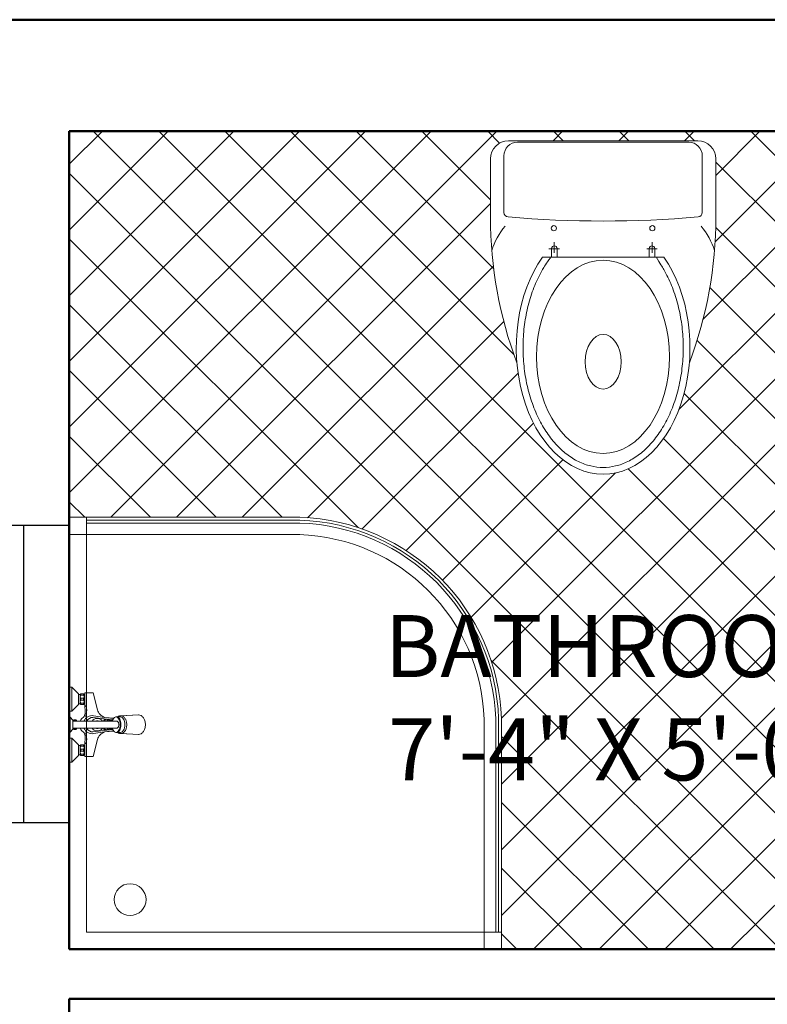
# Model space of a CAD drawing. Units: inches. Extents: x -466983 to 1020, y 324 to 318697.
# Tile 97 of 97: x 810 to 870, y 1006 to 1085. Entities that reach past the tile are written whole.
import ezdxf

# ---------------------------------------------------------------- set-up
doc = ezdxf.new("R2010")
doc.units = ezdxf.units.IN
doc.header["$MEASUREMENT"] = 0
for name, color, linetype, lineweight in [('A-AREA-IDEN', 7, 'Continuous', 25), ('A-FLOR-FIXT', 9, 'Continuous', 18), ('A-FLOR-PATT', 252, 'Continuous', 13), ('A-GLAZ', 4, 'Continuous', 25), ('A-WALL', 7, 'Continuous', 50)]:
    doc.layers.add(name, color=color, linetype=linetype, lineweight=lineweight)
doc.styles.get("Standard").update_dxf_attribs({"font": 'arial.ttf'})

# ---------------------------------------------------------------- blocks, each defined once
blk = doc.blocks.new('Ventilator')
for p, q in [((1433.5927409432, 801.6799676286266), (1457.592740943201, 801.6799676286266)), ((1433.5927409432, 792.6799676286266), (1433.5927409432, 801.6799676286266)), ((1457.592740943201, 801.6799676286266), (1457.592740943201, 792.6799676286266)), ((1433.5927409432, 797.9799676286265), (1457.592740943201, 797.9799676286265)), ((1457.592740943201, 796.3799676286266), (1433.5927409432, 796.3799676286266)), ((1457.592740943201, 792.6799676286266), (1433.5927409432, 792.6799676286266))]:
    blk.add_line(p, q)
blk = doc.blocks.new('B1')
for p, q in [((0, 1300.000000000277), (693.3333333334303, 1300.000000000277)), ((0, 1.023182e-10), (0, 1300.000000000277)), ((52.00000000000727, 52.00000000000045), (52.00000000000727, 1300.000000000277)), ((52.00000000000727, 1291.33333333362), (693.3333333334303, 1291.33333333362)), ((52.00000000000727, 1282.666666666948), (693.3333333334303, 1282.666666666948)), ((0, 1248.000000000277), (693.3333333334303, 1248.000000000277)), ((21.99999999999818, 689.0000000001346), (21.99999999999818, 687.0000000001382)), ((140.3876720592416, 699.4289321882679), (154.4144116848583, 699.4289321882679)), ((208.8876720592416, 705.4289321882679), (153.4804125083301, 702.8756022550479)), ((1248.000000000174, 693.6609680139231), (1248.000000000174, 1.023182e-10)), ((1282.666666666846, 693.6609680139231), (1282.666666666846, 52.00000000010231)), ((1291.333333333514, 693.6609680139231), (1291.333333333517, 52.00000000010231)), ((1300.000000000182, 693.6609680139231), (1300.000000000182, 1.023182e-10)), ((21.99999999999818, 663.0000000001382), (21.99999999999818, 665.0000000001309)), ((140.3876720592416, 652.5710678120049), (154.4144116848583, 652.5710678120049)), ((208.8876720592416, 646.5710678120049), (153.5459520445456, 648.976381547378)), ((52.00000000001091, 52.00000000000045), (1300.000000000178, 52.00000000010231)), ((0, 4.547e-13), (1300.000000000182, 1.023182e-10))]:
    blk.add_line(p, q)
for points in [[(0, 775.000000000131), (0, 789.0000000001346), (8, 789.0000000001346)], [(0, 754.0000000001382), (0, 775.000000000131)], [(8, 789.0000000001346), (8, 717.0000000001309)], [(8, 789.0000000001346), (27.99999999999818, 769.0000000001309), (27.99999999999818, 767.0000000001382)], [(8, 717.0000000001309), (0, 717.0000000001309), (0, 754.0000000001382)], [(27.99999999999818, 767.0000000001382), (33.00000000000182, 767.0000000001382)], [(27.99999999999818, 767.0000000001382), (27.99999999999818, 753.0000000001345)], [(27.99999999999818, 739.0000000001382), (27.99999999999818, 753.0000000001345)], [(33.00000000000182, 767.0000000001382), (35, 769.0000000001309), (43, 769.0000000001309), (45.00000000000182, 767.0000000001382)], [(33.00000000000182, 767.0000000001382), (33.00000000000182, 753.0000000001345)], [(35, 765.0000000001345), (33.00000000000182, 762.0000000001346)], [(33.00000000000182, 758.0000000001346), (35, 756.0000000001346), (43, 756.0000000001346), (45.00000000000182, 758.0000000001346)], [(33.00000000000182, 739.0000000001382), (33.00000000000182, 753.0000000001345)], [(33.00000000000182, 748.0000000001382), (35, 750.0000000001346), (43, 750.0000000001346), (45.00000000000182, 748.0000000001382)], [(35, 741.0000000001346), (33.00000000000182, 744.0000000001345)], [(43, 769.0000000001309), (43, 765.0000000001345), (35, 765.0000000001345), (35, 769.0000000001309)], [(35, 756.0000000001346), (35, 753.0000000001345)], [(35, 750.0000000001346), (35, 753.0000000001345)], [(43, 737.0000000001346), (43, 741.0000000001346), (35, 741.0000000001346), (35, 737.0000000001346)], [(43, 765.0000000001345), (45.00000000000182, 763.0000000001382)], [(43, 756.0000000001346), (43, 753.0000000001345)], [(43, 750.0000000001346), (43, 753.0000000001345)], [(43, 741.0000000001346), (45.00000000000182, 743.0000000001346)], [(47, 767.0000000001382), (45.00000000000182, 767.0000000001382)], [(45.00000000000182, 767.0000000001382), (45.00000000000182, 753.0000000001345)], [(45.00000000000182, 739.0000000001382), (45.00000000000182, 753.0000000001345)], [(47, 739.0000000001382), (47, 767.0000000001382)], [(8, 717.0000000001309), (27.99999999999818, 737.0000000001346), (27.99999999999818, 739.0000000001382)], [(27.99999999999818, 739.0000000001382), (33.00000000000182, 739.0000000001382)], [(33.00000000000182, 739.0000000001382), (35, 737.0000000001346), (43, 737.0000000001346), (45.00000000000182, 739.0000000001382)], [(47, 739.0000000001382), (45.00000000000182, 739.0000000001382)], [(47, 728.0000000001345), (47, 739.0000000001382)], [(0, 687.0000000001382), (0, 699.0000000001382)], [(0, 699.0000000001382), (3, 699.0000000001382)], [(0, 665.0000000001309), (0, 687.0000000001382)], [(3, 699.0000000001382), (3, 676.0000000001346)], [(3, 699.0000000001382), (11, 690.0000000001382), (11, 687.0000000001382)], [(11, 687.0000000001382), (11, 676.0000000001346)], [(140.9999999999982, 687.0000000001382), (11, 687.0000000001382)], [(0, 653.0000000001309), (0, 665.0000000001309)], [(0, 653.0000000001309), (3, 653.0000000001309)], [(3, 653.0000000001309), (3, 676.0000000001346)], [(3, 653.0000000001309), (11, 662.000000000131), (11, 665.0000000001309)], [(11, 665.0000000001309), (11, 676.0000000001346)], [(140.9999999999982, 665.0000000001309), (11, 665.0000000001309)], [(133.9221670278657, 656.0563042479444), (133.0620831697051, 656.0563042479444)], [(7.999999999998181, 635.0000000001382), (0, 635.0000000001382), (0, 598.0000000001309)], [(7.999999999998181, 563.0000000001346), (7.999999999998181, 635.0000000001382)], [(7.999999999998181, 635.0000000001382), (27.99999999999818, 615.0000000001345), (27.99999999999818, 613.0000000001346)], [(47, 624.0000000001345), (47, 613.0000000001346)], [(0, 598.0000000001309), (0, 577.0000000001382)], [(27.99999999999818, 613.0000000001346), (27.99999999999818, 599.0000000001382)], [(27.99999999999818, 613.0000000001346), (33.00000000000182, 613.0000000001346)], [(27.99999999999818, 585.0000000001346), (27.99999999999818, 599.0000000001382)], [(33.00000000000182, 613.0000000001346), (35, 615.0000000001345), (42.99999999999818, 615.0000000001345), (45.00000000000182, 613.0000000001346)], [(33.00000000000182, 613.0000000001346), (33.00000000000182, 599.0000000001382)], [(35, 611.0000000001382), (33.00000000000182, 608.0000000001382)], [(33.00000000000182, 604.0000000001346), (35, 602.0000000001382), (42.99999999999818, 602.0000000001382), (45.00000000000182, 604.0000000001346)], [(33.00000000000182, 585.0000000001346), (33.00000000000182, 599.0000000001382)], [(33.00000000000182, 594.0000000001345), (35, 596.0000000001382), (42.99999999999818, 596.0000000001382), (45.00000000000182, 594.0000000001345)], [(42.99999999999818, 615.0000000001345), (42.99999999999818, 611.0000000001382), (35, 611.0000000001382), (35, 615.0000000001345)], [(35, 602.0000000001382), (35, 599.0000000001382)], [(35, 596.0000000001382), (35, 599.0000000001382)], [(42.99999999999818, 611.0000000001382), (45.00000000000182, 609.0000000001346)], [(42.99999999999818, 602.0000000001382), (42.99999999999818, 599.0000000001382)], [(42.99999999999818, 596.0000000001382), (42.99999999999818, 599.0000000001382)], [(45.00000000000182, 613.0000000001346), (45.00000000000182, 599.0000000001382)], [(47, 613.0000000001346), (45.00000000000182, 613.0000000001346)], [(45.00000000000182, 585.0000000001346), (45.00000000000182, 599.0000000001382)], [(47, 613.0000000001346), (47, 585.0000000001346)], [(0, 577.0000000001382), (0, 563.0000000001346), (7.999999999998181, 563.0000000001346)], [(7.999999999998181, 563.0000000001346), (27.99999999999818, 583.000000000131), (27.99999999999818, 585.0000000001346)], [(27.99999999999818, 585.0000000001346), (33.00000000000182, 585.0000000001346)], [(35, 587.0000000001382), (33.00000000000182, 590.0000000001382)], [(33.00000000000182, 585.0000000001346), (35, 583.000000000131), (42.99999999999818, 583.000000000131), (45.00000000000182, 585.0000000001346)], [(42.99999999999818, 583.000000000131), (42.99999999999818, 587.0000000001382), (35, 587.0000000001382), (35, 583.000000000131)], [(42.99999999999818, 587.0000000001382), (45.00000000000182, 589.0000000001309)], [(47, 585.0000000001346), (45.00000000000182, 585.0000000001346)]]:
    blk.add_lwpolyline(points)
blk.add_lwpolyline([(208.8876720592416, 646.5710678120049), (154.6376720593016, 648.9289321882679, -0.1383183006310921), (148.063043746286, 650.7831906028294, -0.0370381408635636), (145.578855038857, 652.5710678120049), (140.3876720592379, 652.5710678120049, -0.1665558057867227), (136.092755137337, 654.0425753596318, -0.0535717192020755), (133.4948936773198, 656.547585930646), (107, 654.0000000001382, 0.2625940722123521), (85, 631.0000000001346), (72, 580.0000000001419), (47, 580.0000000001419), (47, 585.0000000001346), (45.00000000000182, 585.0000000001346), (42.99999999999818, 583.0000000001346), (35, 583.0000000001346), (33.00000000000182, 585.0000000001346), (27.99999999999818, 585.0000000001346), (27.99999999999818, 583.0000000001346), (7.999999999998181, 563.0000000001382), (0, 563.0000000001382), (0, 577.0000000001418), (0, 598.0000000001346), (0, 635.0000000001418), (7.999999999998181, 635.0000000001418), (27.99999999999818, 615.0000000001382), (27.99999999999818, 613.0000000001346), (33.00000000000182, 613.0000000001346), (35, 615.0000000001382), (42.99999999999818, 615.0000000001382), (45.00000000000182, 613.0000000001346), (47, 613.0000000001346), (47, 624.0000000001382, 0.1247866838288863), (46, 648.0000000001382, 0.1501483781683498), (42.00000000000182, 654.0000000001382, -0.1384844099870248), (32.50754085593508, 665.0000000001345), (21.99999999999818, 665.0000000001345), (21.99999999999818, 663.0000000001382, -0.3003468456066685), (11, 662.3397459768711), (11, 662.0000000001346), (3, 653.0000000001345), (0, 653.0000000001345), (0, 665.0000000001345), (0, 687.0000000001382), (0, 699.0000000001418), (3, 699.0000000001418), (11, 690.0000000001382), (10.99999999999636, 689.6602540496569, -0.3003468456580443), (21.99999999999818, 689.0000000001346), (21.99999999999818, 687.0000000001382), (32.50754085593508, 687.0000000001382, -0.138484409987018), (42.00000000000182, 698.0000000001346, 0.1501483781683498), (46, 704.0000000001346, 0.1247866838288863), (47, 728.0000000001382), (47, 739.0000000001382), (45.00000000000182, 739.0000000001382), (43, 737.0000000001382), (35, 737.0000000001382), (33.00000000000182, 739.0000000001382), (27.99999999999818, 739.0000000001382), (27.99999999999818, 737.0000000001382), (8, 717.0000000001346), (0, 717.0000000001346), (0, 754.0000000001382), (0, 775.0000000001346), (0, 789.0000000001382), (8, 789.0000000001382), (27.99999999999818, 769.0000000001345), (27.99999999999818, 767.0000000001382), (33.00000000000182, 767.0000000001382), (35, 769.0000000001345), (43, 769.0000000001345), (45.00000000000182, 767.0000000001382), (47, 767.0000000001382), (47, 772.0000000001346), (72, 772.0000000001346), (85, 721.0000000001382, 0.2625940722123521), (107, 698.0000000001346), (133.494893670435, 695.4524140702815, -0.0535717192022979), (136.092755137337, 697.9574246406409, -0.1665558057868109), (140.3876720592416, 699.4289321882679), (145.7502000114491, 699.4289321882679, -0.0343443404771406), (148.063043746286, 701.07467377371, -0.1383183006298331), (154.6376720592416, 702.9289321882715), (208.8876720591488, 705.4289321882679, -0.1377032461334603), (216.0999264221609, 703.4042378869926, -0.1070360850488126), (223.0298076829695, 696.809397513447, -0.0808015121757586), (227.273223711496, 687.6931912444343, -0.0687078013104136), (228.8876720592398, 676.0000000001382, -0.0687078013104135), (227.273223711496, 664.3068087558385, -0.0808015121757595), (223.0298076829695, 655.1906024868258, -0.107036085048811), (216.0999264221609, 648.5957621132802, -0.1377032461317454)], format="xyb", close=True)
for points in [[(47, 767.0000000001382), (47, 772.0000000001309), (72, 772.0000000001309), (85, 721.0000000001382, 0.2625940722123521), (107, 698.0000000001346), (133.4948936704422, 695.4524140702887, -0.3591123035969264)], [(47, 728.0000000001345, -0.1247866838288863), (46, 704.0000000001346, -0.1501483781683498), (42.00000000000182, 698.0000000001346, 0.138484409987018), (32.50754085593508, 687.0000000001382, 0.7633705308853952)], [(47, 734.0000000001346, -0.2052577019546359), (52, 726.0000000001309, -0.1374236490949136), (49, 701.0000000001346, -5.029096516974528)], [(11, 688.0000000001346, -0.2034527507076884), (11.27314869702968, 688.6434964536201, -0.0971632324952149), (12.46446609406666, 689.4142135625043, -0.0541309211895364), (13.96123847455419, 689.8322469457524, -0.041071521782227), (15.99999999999818, 690.0000000001382, -0.041071521782232), (18.03876152544581, 689.8322469457524, -0.0541309211895581), (19.53553390593333, 689.4142135625043, -0.0971632324952149), (20.72685130297032, 688.6434964536201, -0.2034527507076884), (21, 688.0000000001346, -0.2034527507076693), (20.72685130297032, 687.3565035466526, -0.0379533313060429), (20.29672106629732, 687.0000000001382, -0.0541309211895384)], [(11.70327893370086, 687.0000000001382, -0.0379533313059558), (11.27314869702968, 687.3565035466526, -0.2034527507076722), (11, 688.0000000001346, -0.2034527507076884)], [(11.14357068821118, 689.7415727613479, -0.2958552022276962), (21.99999999999818, 689.0000000001346, -2.290285352134018)], [(106.0000000000018, 698.0000000001346), (73, 703.0000000001382, 0.3410628393219512), (44.19402075297876, 687.0000000001382, 0.987420997957196)], [(71.00000000000182, 698.0000000001346, 0.2653451188970793), (52.73167562087656, 687.0000000001382, 0.6855978624637613)], [(71.00000000000182, 698.0000000001346), (130.3767751999166, 690.0830966401517, -0.389881551935721)], [(109.0000000000018, 693.0000000001382, 0.3394066855219726), (103.0542662941007, 687.0000000001382)], [(105.3371881863113, 687.0000000001382, -0.2701562118716146), (110, 691.0000000001346), (129.6983785438242, 688.2641140912746, -0.3982822486971544)], [(106.0000000000018, 698.0000000001346), (132.9051195245556, 694.7054955685562, -0.3445125279727503)], [(129.2869436463206, 665.0799945585786, 0.0546118951167688), (131.5488372944073, 659.4332431739494, 0.1055200220071626), (136.092755137337, 654.0425753596318, 0.1665558057868128), (140.3876720592416, 652.5710678120049, 0.1665558057868108), (144.6825889811407, 654.0425753596318, 0.1055200220071628), (149.2265068240704, 659.4332431739494, 0.0682582856346859), (151.8562849435693, 666.5533485092964, 0.0544283700167335), (152.8876720592398, 676.0000000001346, 0.0544283700167333), (151.8562849435693, 685.4466514909764, 0.0682582856346864), (149.2265068240704, 692.5667568263307, 0.1055200220071624), (144.6825889811407, 697.9574246406409, 0.1665558057868127), (140.3876720592416, 699.4289321882679, 0.1665558057868109), (136.092755137337, 697.9574246406409, 0.1055200220071607), (131.5488372944073, 692.5667568263307, 0.0538660454735237), (129.3093729212014, 687.0000000001382, 0.0544283700167342)], [(140.9999999999982, 665.0000000001309, 0.130158640187584), (143.919967274478, 665.7732172227988, 0.1064685849763611), (146.6568542494933, 668.2218254070867, 0.0842476149744631), (148.3593095850538, 671.6519929664936, 0.0732806852421333), (149, 676.0000000001346, 0.0732806852421325), (148.3593095850538, 680.3480070337755, 0.0842476149744645), (146.6568542494933, 683.7781745931861, 0.1064685849763632), (143.919967274478, 686.226782777474, 0.1301586401875921), (140.9999999999982, 687.0000000001382, 0.1301586401875932)], [(141.6455361051521, 652.6849517968694, 0.0451764077839428), (142.9034001510663, 652.5710678120049, 0.1665558057868108), (147.1983170729654, 654.0425753596318, 0.1055200220071628), (151.7422349158969, 659.4332431739494, 0.0682582856346859), (154.3720130353958, 666.5533485092964, 0.0544283700167335), (155.4034001510663, 676.0000000001346, 0.0544283700167333), (154.3720130353958, 685.4466514909764, 0.0682582856346864), (151.7422349158969, 692.5667568263307, 0.1055200220071624), (147.1983170729654, 697.9574246406409, 0.1665558057868127), (142.9034001510663, 699.4289321882679, 0.0451764077839423), (141.6455361051521, 699.315048203407, 0.1055200220071607)], [(145.5788550388533, 652.5710678120049, 0.0370381408635636), (148.063043746286, 650.7831906028294, 0.1383183006298338), (154.6376720592416, 648.9289321882679, 0.138318300629834), (161.2123003721917, 650.7831906028294, 0.1070627939593127), (167.5423708158942, 656.8370490962297, 0.0805227312927088), (171.4136097265637, 665.1966168081926, 0.0683531574638633), (172.8876720592398, 675.9289321882679, 0.0683531574638646), (171.4136097265637, 686.6612475683432, 0.0805227312927094), (167.5423708158942, 695.0208152803061, 0.1070627939593105), (161.2123003721917, 701.07467377371, 0.1383183006298341), (154.6376720592416, 702.9289321882715, 0.1383183006298331), (148.063043746286, 701.07467377371, 0.0343443404771406), (145.7502000114491, 699.4289321882679, 0.0805227312927093)], [(154.4144116848583, 652.5710678120049, 0.1665558057868108), (158.7093286067611, 654.0425753596318, 0.1055200220071628), (163.2532464496908, 659.4332431739494, 0.0682582856346859), (165.8830245691897, 666.5533485092964, 0.0544283700167335), (166.9144116848601, 676.0000000001346, 0.0544283700167333), (165.8830245691897, 685.4466514909764, 0.0682582856346864), (163.2532464496908, 692.5667568263307, 0.1055200220071624), (158.7093286067611, 697.9574246406409, 0.1665558057868127), (154.4144116848583, 699.4289321882679, 0.1665558057868109)], [(207.6853336958775, 646.6233249695179, 0.0217212157548433), (208.8876720592416, 646.5710678120049, 0.1377032461317454), (216.0999264221609, 648.5957621132802, 0.107036085048811), (223.0298076829695, 655.1906024868258, 0.0808015121757595), (227.273223711496, 664.3068087558385, 0.0687078013104135), (228.8876720592398, 676.0000000001346, 0.0687078013104136), (227.273223711496, 687.6931912444343, 0.0808015121757586), (223.0298076829695, 696.809397513447, 0.1070360850488126), (216.0999264221609, 703.4042378869926, 0.1377032461317515), (208.8876720592416, 705.4289321882679, 0.0115815460008583), (208.2459469633304, 705.4140658567775, 0.1070360850488107)], [(11, 664.0000000001346, 0.2034527507076884), (11.27314869702968, 663.356503546649, 0.0971632324952149), (12.46446609406666, 662.5857864377649, 0.0541309211895364), (13.96123847455419, 662.1677530545167, 0.041071521782227), (15.99999999999818, 662.000000000131, 0.041071521782232), (18.03876152544581, 662.1677530545167, 0.0541309211895581), (19.53553390593333, 662.5857864377649, 0.0971632324952149), (20.72685130297032, 663.356503546649, 0.2034527507076884), (21, 664.0000000001346, 0.2034527507076693), (20.72685130297032, 664.6434964536202, 0.0379533313062782), (20.29672106629369, 665.0000000001309, 0.0541309211895384)], [(11.70327893370449, 665.0000000001309, 0.0379533313061481), (11.27314869702968, 664.6434964536202, 0.2034527507076722), (11, 664.0000000001346, 0.2034527507076884)], [(11.14357068821118, 662.2584272389249, 0.2958552022276962), (21.99999999999818, 663.0000000001382, 2.290285352134018)], [(47, 624.0000000001345, 0.1247866838288863), (46, 648.0000000001382, 0.1501483781683498), (42.00000000000182, 654.0000000001382, -0.1384844099870248), (32.50754085593508, 665.0000000001309, -0.7633705308853952)], [(106.0000000000018, 654.0000000001382), (73, 649.0000000001345, -0.341062839321959), (44.19402075297876, 665.0000000001309, -0.987420997957196)], [(47, 585.0000000001346), (47, 580.0000000001382), (72, 580.0000000001382), (85, 631.0000000001346, -0.2625940722123521), (107, 654.0000000001382), (132.4235230446356, 656.4445695236572, 0.3591123035969264)], [(71.00000000000182, 654.0000000001382, -0.2653451188970914), (52.73167562087656, 665.0000000001309, -0.6855978624637613)], [(71.00000000000182, 654.0000000001382), (130.3767751999166, 661.9169033601211, 0.389881551935721)], [(109.0000000000018, 659.0000000001309, -0.3394066855220244), (103.0542662941007, 665.0000000001309)], [(105.3371881863113, 665.0000000001309, 0.2701562118716416), (110, 661.0000000001345), (129.6983785438278, 663.7358859089982, 0.3982822486971544)], [(106.0000000000018, 654.0000000001382), (132.9051195245556, 657.2945044317166, 0.3445125279727503)], [(47, 618.0000000001346, 0.2052577019546359), (52, 626.0000000001382, 0.1374236490949136), (49, 651.0000000001382, 5.029096516974528)]]:
    blk.add_lwpolyline(points, format="xyb")
blk.add_circle((182.931355266388, 149.5974501754249), 47.86997641275996)
for centre, radius, start, end in [((672.5535632588981, 672.5422464127919), 610.4684119504776, 1.92774542086775, 88.10320593202876), ((672.5535632588981, 672.5422464127919), 619.1350786171454, 1.92774542086775, 88.10320593202876), ((672.5535632588981, 672.5422464127919), 627.8017452838134, 1.92774542086775, 88.10320593202876), ((672.5535632588981, 672.5422464127919), 575.801745283806, 1.92774542086775, 88.10320593202876), ((84, 676.0000000001346), 19, 35.37654015188604, 144.6234598481139), ((84, 676.0000000001346), 12.00000000000001, 66.44353569094163, 113.5564643090584), ((120.8125, 676.1250000001309), 12.8131097415889, 112.0608994672246, 121.9251013585072), ((123.9999999999982, 676.0000000001346), 13, 64.79528984039216, 122.2042275039623), ((84, 676.0000000001346), 19, 215.376540151886, 324.623459848114), ((84, 676.0000000001346), 12.00000000000001, 246.4435356909416, 293.5564643090584), ((120.8125, 675.8750000001382), 12.8131097415889, 238.0748986414927, 247.9391005327754), ((123.9999999999982, 676.0000000001346), 13, 237.7957724960376, 295.2047101596079)]:
    blk.add_arc(centre, radius, start, end)
blk = doc.blocks.new('A$C005B7AE8')
for p, q in [((0.4599999173160541, 0.7399999669141835), (0.0399999173159813, 0.7399999669141835)), ((0.439999917316527, 0.7369231961274636), (0.0599999173164179, 0.7369231961274636)), ((-8.26839823e-08, 0.6999999669133103), (-8.26839823e-08, 0.5690287834004267)), ((0.0299999173166725, 0.7069231961286278), (0.029999917315763, 0.5811477270617617)), ((0.4699999173162724, 0.7069231961286278), (0.4699999173162724, 0.5811477270617617)), ((0.4999999173160177, 0.6999999669133103), (0.4999999173160177, 0.5690287833785987)), ((0.1415172819179133, 0.4916755243175431), (0.1415172819179133, 0.5154492432702682)), ((0.3584825527150315, 0.4916755243175431), (0.3584825527150315, 0.5154492432702682)), ((0.3846918195813487, 0.4819999669125537), (0.1153080150515962, 0.4819999669125537)), ((0.1298495880610062, 0.5003783992360696), (0.1533971911394474, 0.5003783992360696)), ((0.135565754210802, 0.4819999669125537), (0.135565754210802, 0.5011511907214299)), ((0.1478168830781215, 0.5011511907214299), (0.1478168830781215, 0.4819999669125537)), ((0.3701502465710291, 0.5003783992360696), (0.3466026434934974, 0.5003783992360696)), ((0.3521829515548234, 0.5011511907214299), (0.3521829515548234, 0.4819999669125537)), ((0.3644340804221429, 0.4819999669125537), (0.3644340804221429, 0.5011511907214299))]:
    blk.add_line(p, q)
for centre in [(0.1407590817070741, 0.546016981927096), (0.3592407529249613, 0.546016981927096)]:
    blk.add_circle(centre, 0.0058207128015492)
for centre, radius, start, end in [((0.0399999173159813, 0.6999999669133103), 0.04, 90, 180), ((0.0599999173164179, 0.7069231961286278), 0.03, 90, 180), ((0.439999917316527, 0.7069231961286278), 0.03, 0, 90), ((0.4599999173160541, 0.6999999669133103), 0.04, 0, 90), ((0.9162347733818023, 0.5697843573143473), 0.9162351676084766, 179.9527510438183, 200.6123382500767), ((0.0399999173159813, 0.5811477270617617), 0.01, 180, 265.0114580301616), ((0.2499999173160177, 2.986999966909934), 2.424999999999394, 265.0114580301616, 274.9885419698384), ((-0.4162349387497671, 0.5697843573143473), 0.9162351676084766, 339.3876617499233, 0.0472489561816761), ((0.4599999173160541, 0.5811477270617617), 0.01, 274.9885419698384, 0), ((0.1538218116911594, 0.4497837234594045), 0.1578971577643038, 140.181504794802, 162.8477667450203), ((0.346178022940876, 0.4497837234594045), 0.1578971577643038, 17.15223325497964, 39.81849520519793), ((0.141691318644007, 0.5005983719747747), 0.0061504591858251, 5.156848388262675, 174.8431516117373), ((0.3583085159880284, 0.5005983719747747), 0.0061504591858251, 5.156848388262675, 174.8431516117373)]:
    blk.add_arc(centre, radius, start, end)
blk.add_ellipse((0.2499999173160177, 0.2809999669116223), major_axis=(4.3e-15, -0.2809999999999999), ratio=0.6859192225533541, start_param=3.915332106759934, end_param=8.65103850759918)
for centre, major_axis, ratio in [((0.2497273054386824, 0.2607283879333408), (4.6e-15, -0.2143896387416461), 0.687861093389952), ((0.2499999173160177, 0.2495750337038771), (4e-16, -0.0607231097518234), 0.6571642650459009)]:
    blk.add_ellipse(centre, major_axis=major_axis, ratio=ratio)
blk.add_open_spline([(0.1330304284401791, 0.4805691871661111), (0.123297561966865, 0.467275065217109), (0.1192040598116364, 0.4608387557527749), (0.1089923119561718, 0.4430896997000673), (0.103240873932009, 0.4312752909245319), (0.0930943572666365, 0.4063656141879619), (0.0886993987696769, 0.3932708291395102), (0.0814055876480779, 0.3661625228414778), (0.0785067868491751, 0.352149423713854), (0.0742960000825406, 0.3235936370911077), (0.0729840366493591, 0.3090513401839416), (0.0719875980385041, 0.2798412472329801), (0.0723031276866095, 0.2651738304266473), (0.0745519352649353, 0.2361210512899561), (0.076485202062031, 0.2217360707581975), (0.0819094268572371, 0.1936478195857489), (0.0854003532995194, 0.1799449487807578), (0.0938301373234936, 0.1536010168056237), (0.0987689237617815, 0.1409603975334903), (0.1099364044266622, 0.1170889910499682), (0.116164929732804, 0.1058587174047716), (0.1297089136187424, 0.0851097239210503), (0.1370239707930523, 0.0755915829504375), (0.152501027386279, 0.0585057705757208), (0.1606621934961367, 0.0509385682526045), (0.1775722209031301, 0.0379140469667618), (0.1863198251348876, 0.0324565718765371), (0.2041561746218576, 0.023724375780148), (0.2132440667546689, 0.0204483489505947), (0.2315630702087219, 0.0160859502211679), (0.2407950771003016, 0.01499791808601), (0.259256859623747, 0.0150020215223776), (0.2684887415816775, 0.0160941591893789), (0.2868071874390807, 0.0204647859718534), (0.2958946431490403, 0.0237449365959037), (0.3137296967424845, 0.0324853214769974), (0.3224764393571604, 0.0379468595056096), (0.3393842548493922, 0.0509792925877264), (0.3475440710253679, 0.058550341942464), (0.3630179485271583, 0.0756434699942474), (0.3703311774997928, 0.0851650790282293), (0.3838710834670564, 0.1059204943594523), (0.3900973596782933, 0.1171537218178855), (0.4012600005589775, 0.1410304195233039), (0.4061961965880983, 0.1536733763350639), (0.4146205471060967, 0.1800212940433994), (0.4181086305634381, 0.1937258131365524), (0.423527009337704, 0.2218166234742966), (0.425457273147913, 0.2362025149268447), (0.4277000090169168, 0.2652563529190957), (0.4280124699726003, 0.2799239176820265), (0.427009923148944, 0.3091335394783528), (0.4256949202253964, 0.3236752172670094), (0.4214781782784485, 0.3522290158871328), (0.4185764618305257, 0.3662407460942632), (0.4112770365782126, 0.3933456040758756), (0.406879379678685, 0.4064383096483653), (0.3967277738520352, 0.4313431800474064), (0.3909739452683425, 0.4431548618158559), (0.380770586511062, 0.4608783582370961), (0.376689084062491, 0.467293849651469), (0.3673029200963356, 0.4823032274071011)], degree=3, knots=[3.915332106759953, 3.915332106759953, 3.915332106759953, 3.915332106759953, 4.014440589322762, 4.014440589322762, 4.176504673233075, 4.176504673233075, 4.338568757143389, 4.338568757143389, 4.500632841053702, 4.500632841053702, 4.662696924964015, 4.662696924964015, 4.824761008874329, 4.824761008874329, 4.986825092784642, 4.986825092784642, 5.148889176694956, 5.148889176694956, 5.310953260605269, 5.310953260605269, 5.473017344515582, 5.473017344515582, 5.635081428425896, 5.635081428425896, 5.797145512336209, 5.797145512336209, 5.959209596246522, 5.959209596246522, 6.121273680156836, 6.121273680156836, 6.283337764067149, 6.283337764067149, 6.445401847977462, 6.445401847977462, 6.607465931887776, 6.607465931887776, 6.769530015798089, 6.769530015798089, 6.931594099708402, 6.931594099708402, 7.093658183618716, 7.093658183618716, 7.255722267529029, 7.255722267529029, 7.417786351439342, 7.417786351439342, 7.579850435349656, 7.579850435349656, 7.741914519259969, 7.741914519259969, 7.903978603170283, 7.903978603170283, 8.066042687080596, 8.066042687080596, 8.22810677099091, 8.22810677099091, 8.390170854901225, 8.390170854901225, 8.552234938811539, 8.552234938811539, 8.651038507599205, 8.651038507599205, 8.651038507599205, 8.651038507599205])

msp = doc.modelspace()

# ---------------------------------------------------------------- hatches: boundary and pattern name
at = {"layer": 'A-FLOR-PATT', "transparency": 33554572}
h = msp.add_hatch(dxfattribs=at)
h.set_pattern_fill('ANSI37', color=256, scale=30)
h.set_pattern_definition([(45, (-1212.413693079869, -290.0350025265127), (-2.651650429449553, 2.651650429449553), []), (135, (-1212.413693079869, -290.0350025265127), (-2.651650429449553, -2.651650429449552), [])])
h.paths.add_polyline_path([(901.805677520904, 1075.937732818422), (900.6144036774049, 1075.937732818422), (900.6144036774049, 1065.385628316983), (899.390971271441, 1065.385628316983), (898.0910743401043, 1065.385628316983), (892.8355944880973, 1058.709752245277, -0.2583770168556315), (892.18750428989, 1058.350891982691), (879.9847834232776, 1058.350891982691, -0.2017697719240963), (879.438188978411, 1058.580825279484), (874.0812133730635, 1065.385628316983), (872.7813164417267, 1065.385628316983), (871.5578840357629, 1065.385628316983), (871.5578840357629, 1075.937732818422), (813.8056775209042, 1075.937732818422), (813.8056775209042, 1044.792233318721), (832.3947444543938, 1044.792233318721, -0.3947951267487684), (848.6601780212009, 1028.535584015862), (848.6601780212009, 1009.937732818421), (901.805677520904, 1009.937732818421), (901.805677520904, 1015.937732818421), (901.3056775209042, 1015.937732818421), (871.3056775209039, 1015.937732818421), (871.3056775209039, 1017.250232818421), (871.3344022102003, 1017.250232818421, -0.4014527144963572), (901.3056775209042, 1045.937732818421), (901.805677520904, 1045.937732818421)])
edge = h.paths.add_edge_path(flags=16)
edge.add_line((847.7730719745084, 1068.948588737025), (847.7730719745069, 1073.708823774771))
edge.add_arc((849.2268986539951, 1073.708823774771), 1.453826679487974, 90, 180, ccw=False)
edge.add_line((849.2268986539951, 1075.162650454259), (864.4920787886183, 1075.162650454259))
edge.add_arc((864.4920787886213, 1073.708823774771), 1.453826679487974, 0, 90.00000000012102, ccw=False)
edge.add_line((865.9459054681093, 1073.708823774771), (865.9459054681081, 1069.00351244647))
edge.add_arc((832.6447385074767, 1068.976050591752), 33.30117828385809, -20.61233806670998, 0.04724903539101888, ccw=False)
edge.add_ellipse((856.8594887213083, 1058.479989307073), major_axis=(-2.091e-13, 10.21313242340307), ratio=0.6859192225533502, start_angle=100.00884331843292, end_angle=259.9911566815624, ccw=False)
edge.add_arc((881.0742389351396, 1068.976050591752), 33.30117828385809, 180.0472490354062, 200.6123380667097, ccw=False)
h.paths.add_polyline_path([(853.145578187156, 1066.481532374271), (853.145578187156, 1066.453444752512), (853.1463399851561, 1066.453444752512, 0.4331071439582673), (852.9166149812349, 1066.684892837266), (852.9166149812349, 1066.453444752512), (853.145578187156, 1066.453444752512), (853.145578187156, 1066.481532374489), (853.088019486549, 1066.612171966583, 0.6979386910037918), (852.699540939094, 1066.453444752512), (852.7003027371272, 1066.453444752512), (852.7003027371272, 1066.481532374489), (852.9166149812349, 1067.001204630995), (852.9166149812349, 1066.684892837266, -0.3962543063594317)], flags=0)
h.paths.add_polyline_path([(861.0186747055222, 1066.481532374271), (861.0186747055222, 1066.453444752512), (861.0194365035225, 1066.453444752512, 0.4164039232557909), (860.8023624614146, 1066.684892837265), (860.8023624614146, 1066.453444752512), (861.0186747055222, 1066.453444752512), (861.0186747055222, 1066.481532374489), (860.9671752720659, 1066.605255499379, 0.7133437187663149), (860.5726374574602, 1066.453444752512), (860.5733992554934, 1066.453444752512), (860.5733992554934, 1066.481532374489), (860.8023624614146, 1067.001204630995), (860.8023624614146, 1066.684892837265, -0.3799725304814568)], flags=0)
edge = h.paths.add_edge_path(flags=0)
edge.add_spline(control_points=[(861.1298377106021, 1065.785468371534), (861.4660965533383, 1065.247811229462), (861.613385559155, 1065.016139861057), (861.9832837951076, 1064.373617117607), (862.1924105327118, 1063.944313665492), (862.5613774174725, 1063.039129539609), (862.7212131906668, 1062.56326642291), (862.9865156700853, 1061.578122280975), (863.0919804897928, 1061.068856600952), (863.2452407883674, 1060.031049745086), (863.293035446714, 1059.502522766744), (863.3294736797056, 1058.440879580113), (863.3181170778639, 1057.907777155726), (863.2366033468288, 1056.85179603536), (863.1664466211855, 1056.328931215311), (862.9695120306455, 1055.307951977375), (862.8427353108815, 1054.809852090196), (862.5365466723708, 1053.852219447362), (862.3571373353129, 1053.392702749349), (861.9514237071658, 1052.524888245794), (861.7251255454219, 1052.116609101398), (861.2330086320977, 1051.362239687588), (860.9672044472572, 1051.016170456457), (860.4047960485765, 1050.394909316517), (860.1082220871676, 1050.119734477926), (859.493696255806, 1049.64606200509), (859.1757900615103, 1049.447558762665), (858.5275631429041, 1049.129883644436), (858.197273503909, 1049.010664382187), (857.5314773710529, 1048.851811036626), (857.1959384637446, 1048.812116564677), (856.5249326641573, 1048.811967422545), (856.1893892160524, 1048.851512676201), (855.5235728169741, 1049.010066967686), (855.1932673158994, 1049.129136347874), (854.5449932971788, 1049.446513839261), (854.2270557868354, 1049.644869411481), (853.6124495619564, 1050.118254324803), (853.3158265363004, 1050.393289340464), (852.7533025914207, 1051.014284587242), (852.487431959371, 1051.360227769297), (851.9951668313728, 1052.114363776776), (851.7687869247744, 1052.522535562859), (851.3628973914427, 1053.390157753425), (851.1833939042357, 1053.849589492002), (850.8770077813263, 1054.807077270704), (850.7501277313783, 1055.30511724975), (850.5529806633081, 1056.326003473117), (850.4827147921034, 1056.848835185142), (850.4009803807432, 1057.904777820697), (850.3895122452288, 1058.437874867502), (850.425728471152, 1059.499535178563), (850.4734126571939, 1060.02808465918), (850.6264565107679, 1061.065963770327), (850.7318153592672, 1061.575279204679), (850.9969137893603, 1062.560548677974), (851.1566514873134, 1063.036487374614), (851.525433403113, 1063.94184619004), (851.7344732542367, 1064.371248757046), (852.1056260411488, 1065.016350037675), (852.2544071072941, 1065.250281998093), (852.608154630964, 1065.733465727338)], knot_values=[3.915332106759953, 3.915332106759953, 3.915332106759953, 3.915332106759953, 4.013467662305501, 4.013467662305501, 4.175531746215815, 4.175531746215815, 4.337595830126129, 4.337595830126129, 4.499659914036444, 4.499659914036444, 4.661723997946757, 4.661723997946757, 4.82378808185707, 4.82378808185707, 4.985852165767384, 4.985852165767384, 5.147916249677697, 5.147916249677697, 5.30998033358801, 5.30998033358801, 5.472044417498324, 5.472044417498324, 5.634108501408637, 5.634108501408637, 5.79617258531895, 5.79617258531895, 5.958236669229264, 5.958236669229264, 6.120300753139577, 6.120300753139577, 6.282364837049891, 6.282364837049891, 6.444428920960204, 6.444428920960204, 6.606493004870517, 6.606493004870517, 6.768557088780831, 6.768557088780831, 6.930621172691144, 6.930621172691144, 7.092685256601457, 7.092685256601457, 7.254749340511771, 7.254749340511771, 7.416813424422084, 7.416813424422084, 7.578877508332397, 7.578877508332397, 7.740941592242711, 7.740941592242711, 7.903005676153024, 7.903005676153024, 8.065069760063338, 8.065069760063338, 8.22713384397365, 8.22713384397365, 8.389197927883965, 8.389197927883965, 8.551262011794279, 8.551262011794279, 8.650370494357087, 8.650370494357087, 8.650370494357087, 8.650370494357087], degree=3, periodic=0)
edge.add_line((852.6421178657537, 1065.785468371534), (861.1298377106024, 1065.785468371534))
edge = h.paths.add_edge_path(flags=0)
edge.add_ellipse((856.8495804607978, 1057.743205248224), major_axis=(-3.1e-13, 7.792134415209829), ratio=0.6878610933899516, start_angle=0, end_angle=360)
h.paths.add_polyline_path([(848.8634419841151, 1069.389059844444), (848.863441984139, 1073.960453158315, -0.4142135623709757), (849.9538119937549, 1075.050823167924), (863.765165448898, 1075.050823167924, -0.4142135623721942), (864.8555354585106, 1073.960453158308), (864.8555354584933, 1069.389059844444, -0.3889362887010341), (864.5236837164459, 1069.026979909221, -0.0435607626104464), (849.19529372618, 1069.02697990933, -0.3889362886276668)], flags=0)
h.paths.add_polyline_path([(853.1006153779753, 1068.112209480768, -1), (852.677499999749, 1068.112209480768, -1)], flags=0)
edge = h.paths.add_edge_path(flags=0)
edge.add_ellipse((856.8594887213083, 1057.33782914961), major_axis=(7.74e-14, 2.20702192546696), ratio=0.6571642650458812, start_angle=0, end_angle=360)
h.paths.add_polyline_path([(861.0414774428674, 1068.112209480768, -1), (860.6183620646412, 1068.112209480768, -1)], flags=0)
edge = h.paths.add_edge_path()
edge.add_line((573.9536545579417, 1057.341203598636), (573.9536545579417, 1075.937732818422))
edge.add_line((573.9536545579417, 1075.937732818422), (558.7307922536265, 1075.937732818422))
edge.add_line((558.7307922536265, 1075.937732818422), (558.7307922536265, 1065.385628316983))
edge.add_line((558.7307922536265, 1065.385628316983), (557.5073598476627, 1065.385628316983))
edge.add_line((557.5073598476627, 1065.385628316983), (556.207462916326, 1065.385628316983))
edge.add_line((556.207462916326, 1065.385628316983), (550.9519830643189, 1058.709752245277))
edge.add_arc((550.3038928661116, 1059.115537236419), 0.7646452537275144, 270, 327.94831933647396, ccw=False)
edge.add_line((550.3038928661116, 1058.350891982691), (538.1011719994992, 1058.350891982691))
edge.add_arc((538.1011719994992, 1059.115537236419), 0.7646452537275137, 224.3704013916024, 270, ccw=False)
edge.add_line((537.5545775546327, 1058.580825279484), (532.1976019492852, 1065.385628316983))
edge.add_line((532.1976019492852, 1065.385628316983), (530.8977050179485, 1065.385628316983))
edge.add_line((530.8977050179485, 1065.385628316983), (529.6742726119846, 1065.385628316983))
edge.add_line((529.6742726119846, 1065.385628316983), (529.6742726119846, 1075.937732818422))
edge.add_line((529.6742726119846, 1075.937732818422), (520.8056775209042, 1075.937732818422))
edge.add_line((520.8056775209042, 1075.937732818422), (520.8056775209042, 1045.937732818422))
edge.add_line((520.8056775209042, 1045.937732818422), (521.3056775209044, 1045.937732818422))
edge.add_arc((521.3056775209042, 1015.937732818422), 30.00000000000023, 2.507490703587223, 89.99999999999977, ccw=False)
edge.add_line((551.2769528316082, 1017.250232818422), (551.3056775209045, 1017.250232818422))
edge.add_line((551.3056775209045, 1017.250232818422), (551.3056775209045, 1015.937732818422))
edge.add_line((551.3056775209045, 1015.937732818422), (520.8056775209042, 1015.937732818422))
edge.add_line((520.8056775209042, 1015.937732818422), (520.8056775209042, 1009.937732818421))
edge.add_line((520.8056775209042, 1009.937732818421), (559.1912990237018, 1010.402158339383))
edge.add_arc((559.1912990237018, 1011.855985018871), 1.453826679487974, 180, 270, ccw=False)
edge.add_line((557.7374723442138, 1011.855985018871), (557.7374723442151, 1016.561296347171))
edge.add_arc((591.0386393048469, 1016.58875820189), 33.3011782838587, 159.3876619332891, 180.0472490353913, ccw=False)
edge.add_ellipse((566.8238890910148, 1027.084819486569), major_axis=(-3.171e-13, 10.21313242340307), ratio=0.6859192225533445, start_angle=280.00884331843395, end_angle=439.99115668156304, ccw=False)
edge.add_arc((542.6091388771833, 1016.58875820189), 33.3011782838584, 0.04724903544490644, 20.612338066710322, ccw=False)
edge.add_line((575.9103058378148, 1016.61622005664), (575.910305837816, 1011.855985018871))
edge.add_arc((574.4564791583282, 1011.855985018871), 1.453826679487974, -90, 0, ccw=False)
edge.add_line((574.4564791583282, 1010.402158339383), (608.8056775209044, 1009.937732818421))
edge.add_line((608.8056775209044, 1009.937732818421), (608.8056775209044, 1041.08570985546))
edge.add_line((608.8056775209044, 1041.08570985546), (590.2179319406538, 1041.08570985546))
edge.add_arc((590.7750219589672, 1057.907380652626), 16.83089295601249, 181.9277454211679, 268.1032059320871, ccw=False)
edge = h.paths.add_edge_path()
edge.add_ellipse((494.2443328575609, 583.6203939656394), major_axis=(-2.099e-13, 10.21313242340307), ratio=0.6859192225533391, start_angle=280.0088433184392, end_angle=439.99115668155895, ccw=False)
edge.add_arc((470.0295826437295, 573.1243326809605), 33.30117828385828, 0.047249035653180727, 20.612338066711573, ccw=False)
edge.add_line((503.3307496043607, 573.1517945358311), (503.3307496043621, 568.3915594979414))
edge.add_arc((501.8769229248741, 568.3915594979414), 1.453826679487974, -90, 0, ccw=False)
edge.add_line((501.8769229248741, 566.9377328184536), (539.8056775209043, 566.9377328184218))
edge.add_line((539.8056775209043, 566.9377328184218), (539.8056775209043, 572.9377328184218))
edge.add_line((539.8056775209043, 572.9377328184218), (539.3056775209043, 572.9377328184218))
edge.add_line((539.3056775209043, 572.9377328184218), (509.3056775209042, 572.9377328184218))
edge.add_line((509.3056775209042, 572.9377328184218), (509.3056775209042, 574.2502328184218))
edge.add_line((509.3056775209042, 574.2502328184218), (509.3344022102004, 574.2502328184218))
edge.add_arc((539.3056775209043, 572.9377328184218), 30.00000000000003, 90, 177.4925092964128, ccw=False)
edge.add_line((539.3056775209043, 602.9377328184218), (539.8056775209043, 602.9377328184218))
edge.add_line((539.8056775209043, 602.9377328184218), (539.8056775209043, 626.9377328184219))
edge.add_line((539.8056775209043, 626.9377328184219), (531.7718318056131, 626.9377328184219))
edge.add_line((531.7718318056131, 626.9377328184219), (531.7718318056131, 616.3856283169836))
edge.add_line((531.7718318056131, 616.3856283169836), (530.5483993996492, 616.3856283169836))
edge.add_line((530.5483993996492, 616.3856283169836), (529.2485024683125, 616.3856283169836))
edge.add_line((529.2485024683125, 616.3856283169836), (523.7105154427977, 609.3508919826913))
edge.add_line((523.7105154427977, 609.3508919826913), (510.7766285267865, 609.3508919826913))
edge.add_line((510.7766285267865, 609.3508919826913), (505.2386415012717, 616.3856283169835))
edge.add_line((505.2386415012717, 616.3856283169835), (503.9387445699351, 616.3856283169836))
edge.add_line((503.9387445699351, 616.3856283169836), (502.7153121639711, 616.3856283169836))
edge.add_line((502.7153121639711, 616.3856283169836), (502.7153121639712, 626.9377328184219))
edge.add_line((502.7153121639712, 626.9377328184219), (481.698294634846, 626.937732818422))
edge.add_line((481.698294634846, 626.937732818422), (481.6982946348461, 610.9950036909872))
edge.add_arc((467.2703297247223, 611.4728203914133), 14.43587476556121, 271.9277454211847, 358.103205932099, ccw=False)
edge.add_line((467.7559403853078, 597.0451157044822), (451.8056775209041, 597.0451157044822))
edge.add_line((451.8056775209041, 597.0451157044822), (451.8056775209041, 584.4035114605515))
edge.add_line((451.8056775209041, 584.4035114605515), (451.8056775209043, 566.9377328184218))
edge.add_line((451.8056775209043, 566.9377328184218), (486.6117427902477, 566.9377328184536))
edge.add_arc((486.6117427902477, 568.3915594979414), 1.453826679487974, 180, 270, ccw=False)
edge.add_line((485.1579161107598, 568.3915594979414), (485.157916110761, 573.0968708261933))
edge.add_arc((518.4590830713927, 573.1243326809608), 33.3011782838585, 159.387661933289, 180.0472490354759, ccw=False)
h.paths.add_polyline_path([(836.2608886421394, 1020.732838196592), (879.8898108795202, 1020.732838196592), (879.8898108795202, 1039.390182443977), (836.2608886421394, 1039.390182443977)], flags=25)
h.paths.add_polyline_path([(549.9851009445293, 1036.749159167106), (593.6140231819099, 1036.749159167106), (593.6140231819099, 1055.406503414491), (549.9851009445293, 1055.406503414491)], flags=24)
h.paths.add_polyline_path([(475.1230325221868, 595.5958681380167), (518.7519547595675, 595.5958681380167), (518.7519547595675, 614.2532123854019), (475.1230325221868, 614.2532123854019)], flags=24)

# ---------------------------------------------------------------- linework, layer by layer
at = {"layer": 'A-WALL'}
for p, q in [((391.8056775209043, 1084.937732818421), (991.8056775209043, 1084.937732818421)), ((813.8056775209042, 1075.937732818422), (813.8056775209042, 1009.937732818422)), ((813.8056775209042, 1075.937732818422), (982.805677520904, 1075.937732818422)), ((901.805677520904, 1009.937732818421), (813.8056775209042, 1009.937732818421)), ((929.8056775209042, 1005.937732818421), (813.8056775209042, 1005.937732818422)), ((813.8056775209042, 1005.937732818422), (813.8056775209044, 870.9377328184215))]:
    msp.add_line(p, q, dxfattribs=at)

# ---------------------------------------------------------------- block references
at = {"layer": 'A-FLOR-FIXT'}
for name, p, xscale, yscale, zscale in [('A$C005B7AE8', (847.7730749797128, 1048.26685808629), 36.34566698719936, 36.34566698719936, 36.34566698719936), ('B1', (813.8056775209042, 1009.937732818421), 0.0268111542309937, 0.0268111542309937, 0.0268111542309937)]:
    msp.add_blockref(name, p, dxfattribs=dict(at, xscale=xscale, yscale=yscale, zscale=zscale))
at = {"layer": 'A-GLAZ', "rotation": 270}
msp.add_blockref('Ventilator', (12.12570989227788, 2477.73988799651), dxfattribs=at)

# ---------------------------------------------------------------- texts
at = {"layer": 'A-AREA-IDEN', "insert": (823.1222914307581, 1036.902119688179), "char_height": 5, "attachment_point": 1}
msp.add_mtext_dynamic_manual_height_columns('\\pxqc;{\\fArial|b1|i0|c0|p34;BATHROOM\\P7\'-4" X 5\'-0"}', width=69.92316986614605, gutter_width=1, heights=[0], dxfattribs=at)

doc.saveas('drawing.dxf')
